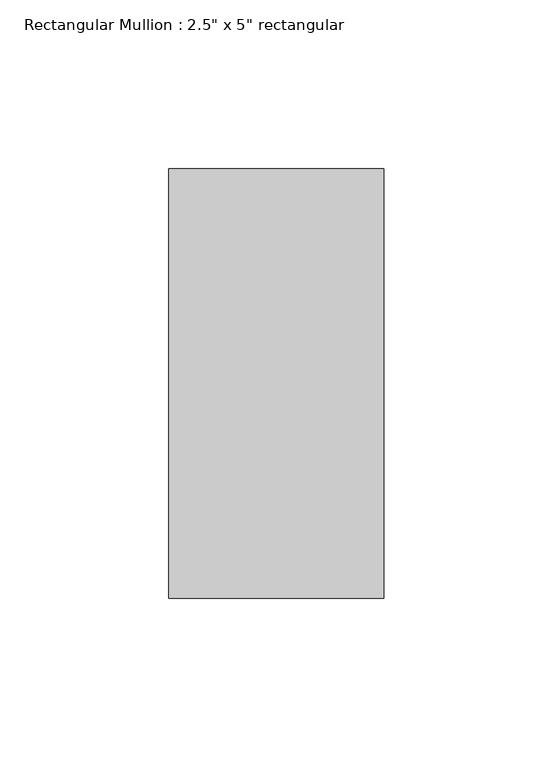
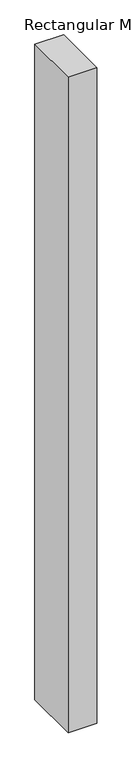
"""IFC4 building model written with IfcOpenShell, lengths in millimetres: member geometry."""

from ifc_helpers import new_model, si_unit, frame, origin, place, context, project, spatial, polyline, outline, extrude, source, transform, mapped, element, save


def member_bcb10b1d(model_context):
    return source(origin(), model_context, "Body", "SweptSolid", [
        extrude(outline(polyline([(0.0, 63.5), (0.0, -63.5), (-63.5, -63.5), (-63.5, 63.5), (0.0, 63.5)])), frame((0.0, 0.0, -1529.8884341), z_axis=(0.0, 0.0, 1.0), x_axis=(1.0, 0.0, 0.0)), (0.0, 0.0, 1.0), 1529.8884341),
    ])


if __name__ == "__main__":
    model = new_model("IFC4")
    model_context = context("Model", 3, world=origin())
    ifc_project = project(units=[si_unit("LENGTHUNIT", "METRE", prefix="MILLI")], contexts=[model_context])
    site = spatial("IfcSite", under=ifc_project)
    building = spatial("IfcBuilding", under=site)
    placement = place(None, origin())
    member_shape = member_bcb10b1d(model_context)
    element("IfcMember", 1, ObjectType="Rectangular Mullion : 2.5\" x 5\" rectangular", at=placement, inside=building, context=model_context, shape_type="MappedRepresentation", body=[
        mapped(member_shape, transform((0.0, 0.0, 0.0), x_axis=(1.0, 0.0, 0.0), y_axis=(0.0, 1.0, 0.0), z_axis=(0.0, 0.0, 1.0))),
    ])
    save(model, "model.ifc")

# Revit data of these elements
# Type "Rectangular Mullion : 2.5\" x 5\" rectangular"
#   built-in parameter 1007304 = 0.416667 (stored number, unit not read)
#   built-in parameter 1007301 = 0.104167 (stored number, unit not read)
#   built-in parameter 1007300 = 0.104167 (stored number, unit not read)
# Element 1 (IfcMember, "Rectangular Mullion : 2.5\" x 5\" rectangular")
#   Materials on its faces: "Aluminum"
# Materials
#   "Aluminum": class "Metal", colour RGB 247 247 247, transparency 0, Description = "Aluminum 6061", Cost = 0
